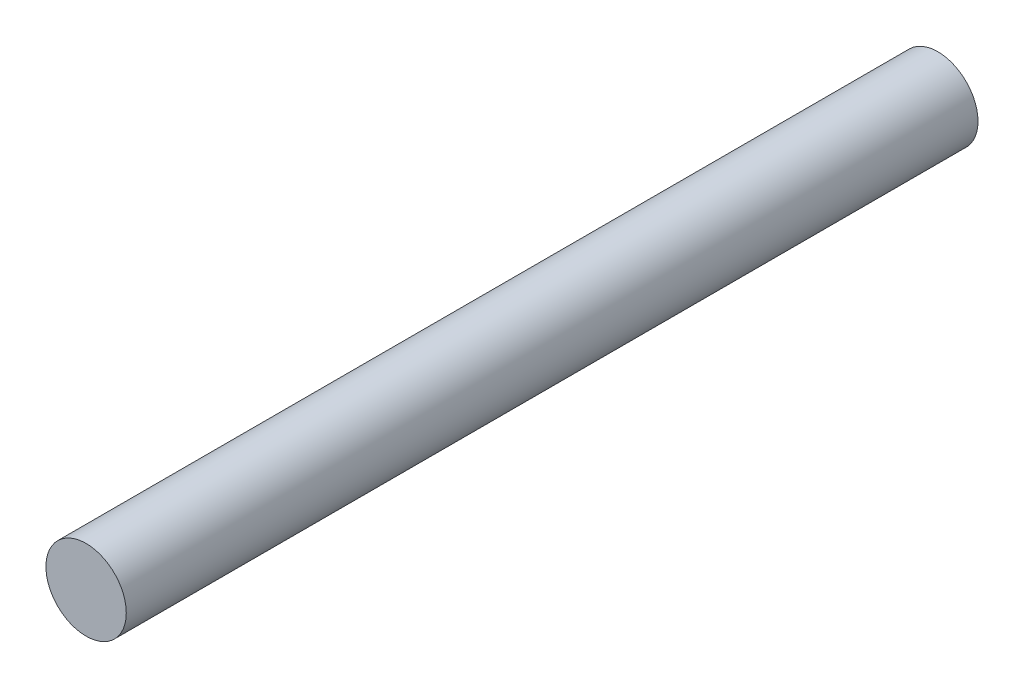
SolidWorks part; units mm, degrees
material "Plain Carbon Steel"
ref_plane "Front Plane" through (0, 0, 0) normal (0, 0, 1) x (1, 0, 0)
ref_plane "Top Plane" through (0, 0, 0) normal (0, 1, 0) x (1, 0, 0)
ref_plane "Right Plane" through (0, 0, 0) normal (1, 0, 0) x (0, 0, -1)
sketch "Rod Profile Ø5" plane through (0, 0, 0) normal (0, 0, 1) x (1, 0, 0)
  circle A0 centre (0, 0) radius 2.5
  dimension "D1" = 5
extrude "Rod Body L53" add sketch "Rod Profile Ø5" along normal mid plane 53
